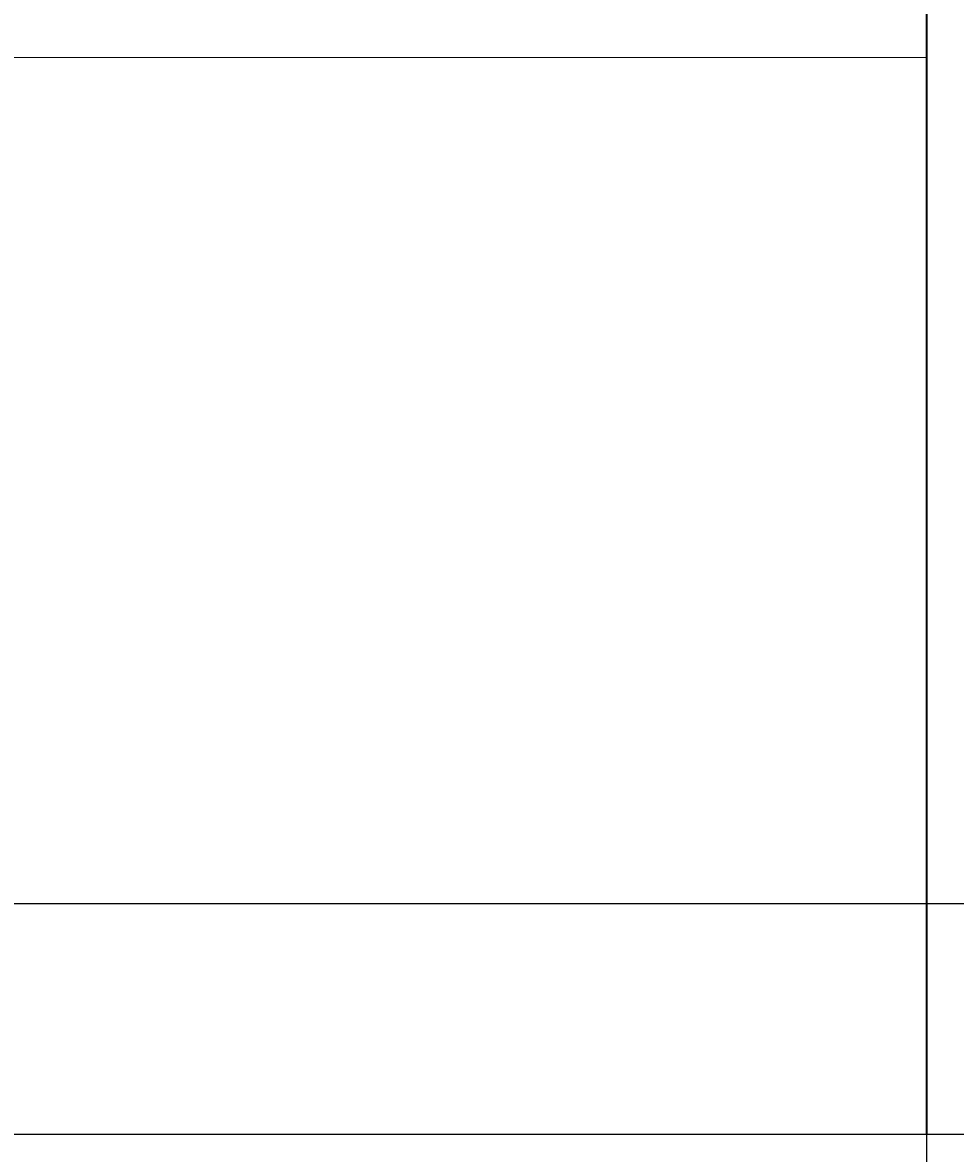
# Model space of a CAD drawing. Units: feet. Extents: x 1654 to 2985, y 1348 to 2230.
# Tile 20 of 53: x 2167 to 2203, y 1565 to 1609. Entities that reach past the tile are written whole.
import ezdxf

# ---------------------------------------------------------------- set-up
doc = ezdxf.new("R2010")
doc.units = ezdxf.units.FT
for name, color, linetype, lineweight in [('A-ANNO-DIMS', 2, 'Continuous', 18), ('A-FLOR', 7, 'Continuous', 25), ('A-FLOR-STRS', 7, 'Continuous', 18), ('A-WALL', 7, 'Continuous', 35)]:
    doc.layers.add(name, color=color, linetype=linetype, lineweight=lineweight)
doc.styles.get("Standard").update_dxf_attribs({"font": 'arial.ttf'})
doc.dimstyles.get("Standard").update_dxf_attribs({"dimtxt": 0.18, "dimasz": 0.18, "dimexe": 0.18, "dimexo": 0.0625, "dimgap": 0.09, "dimtad": 0, "dimtih": 1, "dimtoh": 1, "dimdec": 4, "dimzin": 0, "dimdsep": 46, "dimtxsty": 'Standard', "dimcen": 0.09, "dimadec": 0, "dimazin": 0, "dimtfac": 1, "dimtdec": 4, "dimtofl": 0, "dimtmove": 0, "dimatfit": 3, "dimfxl": 1, "dimtolj": 1, "dimtzin": 0, "dimarcsym": 0})

# ---------------------------------------------------------------- blocks, each defined once
blk = doc.blocks.new('STAIR-RETURN')
blk.add_line((0, 42), (72, 42))
blk = doc.blocks.new('*D72')
at = {"layer": 'A-ANNO-DIMS', "color": 0, "lineweight": -2, "transparency": 16777216}
for p, q in [((2202.155, 1751.255), (2230.172, 1751.255)), ((2229.992, 1751.075), (2229.992, 1658.438)), ((2229.992, 1565.435), (2229.992, 1658.072)), ((2202.155, 1565.255), (2230.172, 1565.255))]:
    blk.add_line(p, q, dxfattribs=at)
at = {"layer": 'A-ANNO-DIMS', "color": 0, "transparency": 16777216}
for points in [[(2229.962, 1751.075), (2230.022, 1751.075), (2229.992, 1751.255)], [(2229.962, 1565.435), (2230.022, 1565.435), (2229.992, 1565.255)]]:
    blk.add_solid(points, dxfattribs=at)
at = {"layer": 'Defpoints', "color": 0, "transparency": 16777216}
for p in [(2202.092, 1751.255), (2229.992, 1751.255), (2202.092, 1565.255)]:
    blk.add_point(p, dxfattribs=at)
at = {"layer": 'A-ANNO-DIMS', "color": 0, "transparency": 16777216, "insert": (2229.992, 1658.255), "char_height": 0.18, "attachment_point": 5}
blk.add_mtext('\\A1;STAIR 186 TYP.', dxfattribs=at)
blk = doc.blocks.new('*D73')
at = {"layer": 'A-ANNO-DIMS', "color": 0, "lineweight": -2, "transparency": 16777216}
for p, q in [((2130.092, 1565.192), (2130.092, 1537.175)), ((2202.092, 1565.192), (2202.092, 1537.175)), ((2130.272, 1537.355), (2165.565, 1537.355)), ((2201.912, 1537.355), (2166.62, 1537.355))]:
    blk.add_line(p, q, dxfattribs=at)
at = {"layer": 'A-ANNO-DIMS', "color": 0, "transparency": 16777216}
for points in [[(2130.272, 1537.385), (2130.272, 1537.325), (2130.092, 1537.355)], [(2201.912, 1537.385), (2201.912, 1537.325), (2202.092, 1537.355)]]:
    blk.add_solid(points, dxfattribs=at)
at = {"layer": 'Defpoints', "color": 0, "transparency": 16777216}
for p in [(2130.092, 1565.255), (2202.092, 1565.255), (2202.092, 1537.355)]:
    blk.add_point(p, dxfattribs=at)
at = {"layer": 'A-ANNO-DIMS', "color": 0, "transparency": 16777216, "insert": (2166.092, 1537.355), "char_height": 0.18, "attachment_point": 5}
blk.add_mtext('\\A1;72 TYP.', dxfattribs=at)
blk = doc.blocks.new('*D80')
at = {"layer": 'A-ANNO-DIMS', "color": 0, "lineweight": -2, "transparency": 16777216}
for p, q in [((2070.092, 2039.192), (2070.092, 1534.075)), ((2202.092, 2039.192), (2202.092, 1534.075)), ((2070.272, 1534.255), (2135.813, 1534.255)), ((2201.912, 1534.255), (2136.372, 1534.255))]:
    blk.add_line(p, q, dxfattribs=at)
at = {"layer": 'A-ANNO-DIMS', "color": 0, "transparency": 16777216}
for points in [[(2070.272, 1534.285), (2070.272, 1534.225), (2070.092, 1534.255)], [(2201.912, 1534.285), (2201.912, 1534.225), (2202.092, 1534.255)]]:
    blk.add_solid(points, dxfattribs=at)
at = {"layer": 'Defpoints', "color": 0, "transparency": 16777216}
for p in [(2070.092, 2039.255), (2202.092, 2039.255), (2202.092, 1534.255)]:
    blk.add_point(p, dxfattribs=at)
at = {"layer": 'A-ANNO-DIMS', "color": 0, "transparency": 16777216, "insert": (2136.092, 1534.255), "char_height": 0.18, "attachment_point": 5}
blk.add_mtext('\\A1;132', dxfattribs=at)
blk = doc.blocks.new('*D90')
at = {"layer": 'A-ANNO-DIMS', "color": 0, "lineweight": -2, "transparency": 16777216}
for p, q in [((1852.155, 1641.187), (2242.272, 1641.187)), ((2242.092, 1641.007), (2242.092, 1607.903)), ((2242.092, 1574.435), (2242.092, 1607.539)), ((1852.155, 1574.255), (2242.272, 1574.255))]:
    blk.add_line(p, q, dxfattribs=at)
at = {"layer": 'A-ANNO-DIMS', "color": 0, "transparency": 16777216}
for points in [[(2242.062, 1641.007), (2242.122, 1641.007), (2242.092, 1641.187)], [(2242.062, 1574.435), (2242.122, 1574.435), (2242.092, 1574.255)]]:
    blk.add_solid(points, dxfattribs=at)
at = {"layer": 'Defpoints', "color": 0, "transparency": 16777216}
for p in [(1852.092, 1641.187), (2242.092, 1641.187), (1852.092, 1574.255)]:
    blk.add_point(p, dxfattribs=at)
at = {"layer": 'A-ANNO-DIMS', "color": 0, "transparency": 16777216, "insert": (2242.092, 1607.721), "char_height": 0.18, "attachment_point": 5}
blk.add_mtext('\\A1;66.93', dxfattribs=at)

msp = doc.modelspace()

# ---------------------------------------------------------------- linework, layer by layer
at = {"layer": 'A-FLOR'}
msp.add_line((2008.0924, 1565.2549), (2211.0924, 1565.2549), dxfattribs=at)
at = {"layer": 'A-WALL'}
msp.add_line((2202.0924, 1742.2549), (2202.0924, 1565.2549), dxfattribs=at)

# ---------------------------------------------------------------- block references
at = {"layer": 'A-FLOR-STRS'}
msp.add_blockref('STAIR-RETURN', (2130.092, 1565.255), dxfattribs=at)

# ---------------------------------------------------------------- dimensions: what is measured, and where the dimension line sits
at = {"layer": 'A-ANNO-DIMS'}
dim = msp.add_linear_dim(base=(2202.0924, 1534.2549), p1=(2070.0924, 2039.2549), p2=(2202.0924, 2039.2549), dimstyle='Standard', override={"dimdec": 0, "dimlfac": 1, "dimrnd": 0, "dimzin": 0, "dimdsep": 46, "dimlunit": 2}, dxfattribs=at)
dim.commit()
dim.dimension.update_dxf_attribs({"geometry": '*D80', "text_midpoint": (2136.0924, 1534.2549)})
dim = msp.add_linear_dim(base=(2229.9924, 1751.2549), p1=(2202.0924, 1565.2549), p2=(2202.0924, 1751.2549), angle=90, text='STAIR <> TYP.', dimstyle='Standard', override={"dimdec": 0, "dimlfac": 1, "dimrnd": 0, "dimzin": 0, "dimdsep": 46, "dimlunit": 2}, dxfattribs=at)
dim.commit()
dim.dimension.update_dxf_attribs({"geometry": '*D72', "text_midpoint": (2229.9924, 1658.2549)})
dim = msp.add_linear_dim(base=(2242.0924, 1641.187), p1=(1852.0924, 1574.2549), p2=(1852.0924, 1641.187), angle=90, dimstyle='Standard', override={"dimdec": 2, "dimlfac": 1, "dimrnd": 0, "dimzin": 0, "dimdsep": 46, "dimlunit": 2}, dxfattribs=at)
dim.commit()
dim.dimension.update_dxf_attribs({"geometry": '*D90', "text_midpoint": (2242.0924, 1607.721)})
dim = msp.add_linear_dim(base=(2202.0924, 1537.3549), p1=(2130.0924, 1565.2549), p2=(2202.0924, 1565.2549), text='<> TYP.', dimstyle='Standard', override={"dimdec": 0, "dimlfac": 1, "dimrnd": 0, "dimzin": 0, "dimdsep": 46, "dimlunit": 2}, dxfattribs=at)
dim.commit()
dim.dimension.update_dxf_attribs({"geometry": '*D73', "text_midpoint": (2166.0924, 1537.3549)})

doc.saveas('drawing.dxf')
